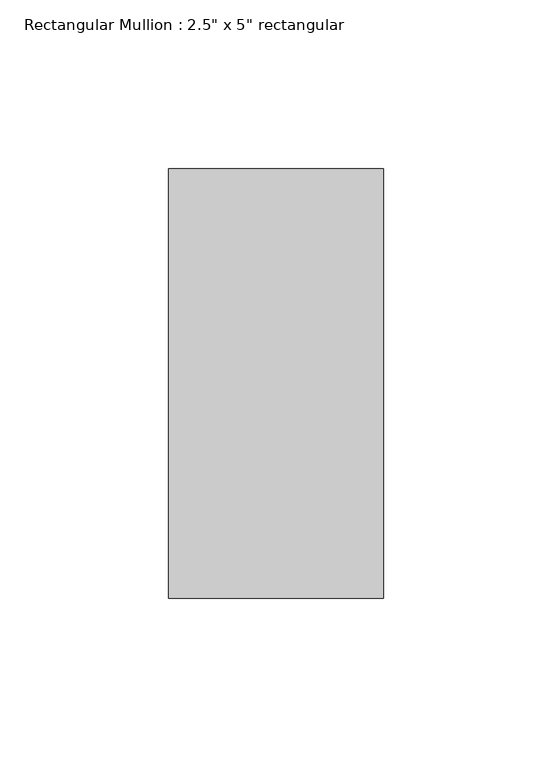
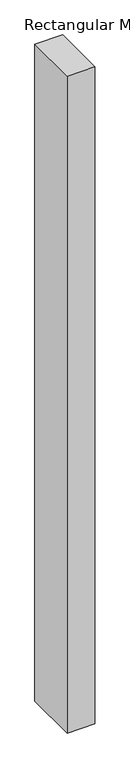
"""IFC4 building model written with IfcOpenShell, lengths in millimetres: member geometry."""

from ifc_helpers import new_model, si_unit, frame, origin, place, context, project, spatial, polyline, outline, extrude, source, transform, mapped, element, save


def member_1d1a2070(model_context):
    return source(origin(), model_context, "Body", "SweptSolid", [
        extrude(outline(polyline([(0.0, 63.5), (0.0, -63.5), (-63.5, -63.5), (-63.5, 63.5), (0.0, 63.5)])), frame((0.0, 0.0, -1582.9994987), z_axis=(0.0, 0.0, 1.0), x_axis=(1.0, 0.0, 0.0)), (0.0, 0.0, 1.0), 1582.9994987),
    ])


if __name__ == "__main__":
    model = new_model("IFC4")
    model_context = context("Model", 3, world=origin())
    ifc_project = project(units=[si_unit("LENGTHUNIT", "METRE", prefix="MILLI")], contexts=[model_context])
    site = spatial("IfcSite", under=ifc_project)
    building = spatial("IfcBuilding", under=site)
    placement = place(None, origin())
    member_shape = member_1d1a2070(model_context)
    element("IfcMember", 1, ObjectType="Rectangular Mullion : 2.5\" x 5\" rectangular", at=placement, inside=building, context=model_context, shape_type="MappedRepresentation", body=[
        mapped(member_shape, transform((0.0, 0.0, 0.0), x_axis=(1.0, 0.0, 0.0), y_axis=(0.0, 1.0, 0.0), z_axis=(0.0, 0.0, 1.0))),
    ])
    save(model, "model.ifc")

# Revit data of these elements
# Type "Rectangular Mullion : 2.5\" x 5\" rectangular"
#   built-in parameter 1007304 = 0.416667 (stored number, unit not read)
#   built-in parameter 1007301 = 0.104167 (stored number, unit not read)
#   built-in parameter 1007300 = 0.104167 (stored number, unit not read)
# Element 1 (IfcMember, "Rectangular Mullion : 2.5\" x 5\" rectangular")
#   Materials on its faces: "Aluminum"
# Materials
#   "Aluminum": class "Metal", colour RGB 247 247 247, transparency 0, Description = "Aluminum 6061", Cost = 0
